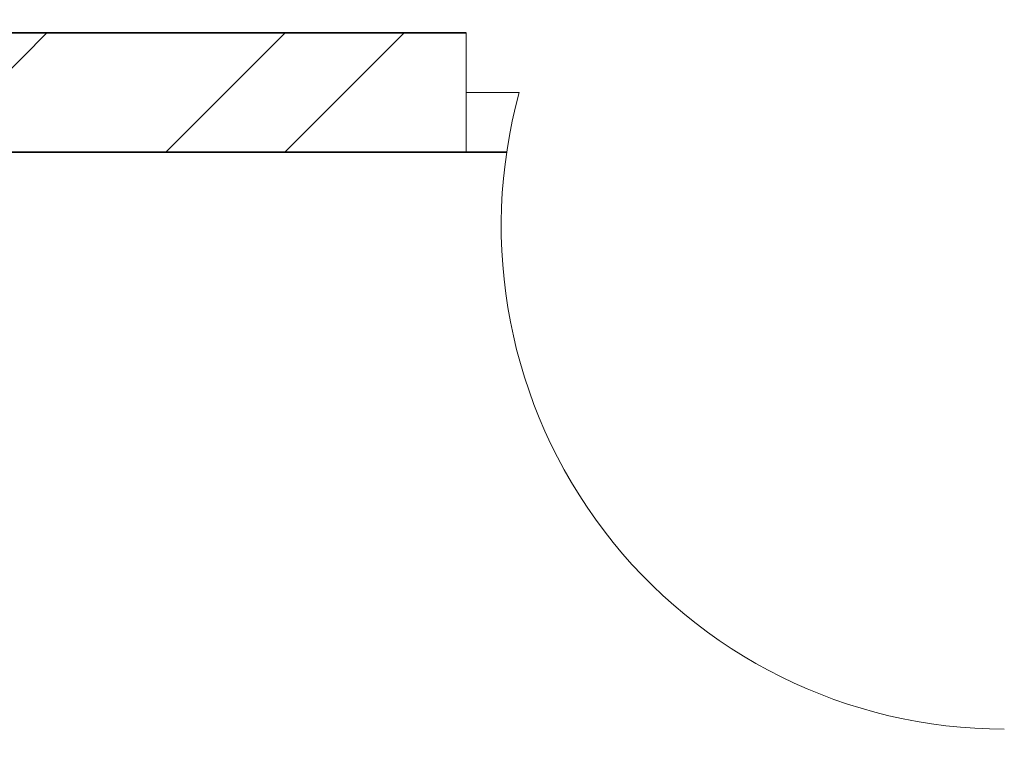
# Model space of a CAD drawing. Units: inches. Extents: x 1885 to 2748, y 783 to 2421.
# Tile 14 of 117: x 2065 to 2102, y 1065 to 1093. Entities that reach past the tile are written whole.
import ezdxf

# ---------------------------------------------------------------- set-up
doc = ezdxf.new("R2010")
doc.units = ezdxf.units.IN
doc.layers.add('A-DOOR', color=31, linetype='Continuous', lineweight=18)
doc.layers.add('A-WALL', color=7, linetype='Continuous', lineweight=35)
doc.layers.add('A-WALL-PATT', color=85, linetype='Continuous', lineweight=13, true_color=0x58ba48)

msp = doc.modelspace()

# ---------------------------------------------------------------- hatches: boundary and pattern name
at = {"layer": 'A-WALL-PATT'}
h = msp.add_hatch(dxfattribs=at)
h.set_pattern_fill('ANSI32', color=256)
h.paths.add_polyline_path([(2007.772, 2318.006), (1980.774, 2318.006), (1980.774, 2281.215), (1985.274, 2281.215), (1985.274, 2313.506), (2007.772, 2313.506), (2007.772, 2315.756)])
h.paths.add_polyline_path([(2094.324, 2318.006), (2067.772, 2318.006), (2067.772, 2313.506), (2094.324, 2313.506), (2094.324, 2315.756)])
h.paths.add_polyline_path([(2131.367, 2315.756), (2131.367, 2318.006), (2131.189, 2318.006), (2112.609, 2318.006), (2112.609, 2313.506), (2117.274, 2313.506), (2117.274, 2255.201), (2121.774, 2255.201), (2121.774, 2313.506), (2131.367, 2313.506)])
h.paths.add_polyline_path([(2190.512, 2318.006), (2155.367, 2318.006), (2155.367, 2313.506), (2169.774, 2313.506), (2169.774, 2229.506), (2121.774, 2229.506), (2121.774, 2233.451), (2119.524, 2233.451), (2117.274, 2233.451), (2117.274, 2201.101), (2121.774, 2201.101), (2121.774, 2225.006), (2169.774, 2225.006), (2169.774, 2165.006), (2306.274, 2165.006), (2306.274, 2066.006), (2310.774, 2066.006), (2344.274, 2066.006), (2486.274, 2066.006), (2486.274, 1886.006), (2483.02, 1886.006), (2483.02, 1881.506), (2486.274, 1881.506), (2486.274, 1880.678), (2490.774, 1880.678), (2490.774, 2070.506), (2344.274, 2070.506), (2310.774, 2070.506), (2310.774, 2165.006), (2310.774, 2173.636), (2308.524, 2173.636), (2306.274, 2173.636), (2306.274, 2169.506), (2174.274, 2169.506), (2174.274, 2313.506), (2190.512, 2313.506), (2190.512, 2315.756)])
h.paths.add_polyline_path([(1985.274, 2221.215), (1980.774, 2221.215), (1980.774, 2165.006), (1992.774, 2165.006), (1992.774, 2141.927), (1997.274, 2141.927), (1997.274, 2165.006), (2117.274, 2165.006), (2117.274, 2163.126), (2121.774, 2163.126), (2121.774, 2172.734), (2119.524, 2172.734), (2117.274, 2172.734), (2117.274, 2169.506), (1985.274, 2169.506)])
h.paths.add_polyline_path([(1997.274, 2105.927), (1992.774, 2105.927), (1992.774, 2070.506), (2016.774, 2070.506), (2016.774, 2059.123), (2019.024, 2059.123), (2021.274, 2059.123), (2021.274, 2070.506), (2117.274, 2070.506), (2117.274, 2022.506), (2114.423, 2022.506), (2114.423, 2018.006), (2123.627, 2018.006), (2123.627, 2020.256), (2123.627, 2022.506), (2121.774, 2022.506), (2121.774, 2142.587), (2119.524, 2142.587), (2117.274, 2142.587), (2117.274, 2075.006), (1997.274, 2075.006)])
h.paths.add_polyline_path([(2092.029, 2020.256), (2092.029, 2022.506), (2021.274, 2022.506), (2021.274, 2035.123), (2016.774, 2035.123), (2016.774, 2018.006), (2016.774, 1978.784), (2021.274, 1978.784), (2021.274, 2018.006), (2092.029, 2018.006)])
h.paths.add_polyline_path([(2260.938, 2022.506), (2153.105, 2022.506), (2153.105, 2020.256), (2153.105, 2018.006), (2155.274, 2018.006), (2155.274, 1886.006), (2107.629, 1886.006), (2107.629, 1881.506), (2182.911, 1881.506), (2182.911, 1883.756), (2182.911, 1886.006), (2159.774, 1886.006), (2159.774, 2018.006), (2260.938, 2018.006), (2260.938, 2020.256)])
h.paths.add_polyline_path([(2047.629, 1883.756), (2047.629, 1886.006), (2021.274, 1886.006), (2021.274, 1918.784), (2019.024, 1918.784), (2016.774, 1918.784), (2016.774, 1881.506), (2047.629, 1881.506)])
h.paths.add_polyline_path([(2306.361, 1883.756), (2306.361, 1886.006), (2296.274, 1886.006), (2296.274, 1982.006), (2316.535, 1982.006), (2316.535, 1984.256), (2316.535, 1986.506), (2296.274, 1986.506), (2296.274, 2022.506), (2289.276, 2022.506), (2289.276, 2018.006), (2291.774, 2018.006), (2291.774, 1886.006), (2242.911, 1886.006), (2242.911, 1881.506), (2306.361, 1881.506)], flags=17)
h.paths.add_polyline_path([(1985.274, 1843.006), (2021.6, 1843.006), (2021.534, 1845.441), (2021.477, 1847.506), (1980.774, 1847.506), (1980.774, 1809.446), (1985.274, 1809.446)])
h.paths.add_polyline_path([(2131.482, 1845.256), (2131.482, 1847.506), (2081.534, 1847.506), (2081.534, 1843.006), (2117.274, 1843.006), (2117.274, 1784.147), (2119.524, 1784.147), (2121.774, 1784.147), (2121.774, 1843.006), (2131.482, 1843.006)])
h.paths.add_polyline_path([(2203.886, 1847.506), (2155.482, 1847.506), (2155.482, 1843.006), (2169.774, 1843.006), (2169.774, 1759.006), (2121.774, 1759.006), (2121.774, 1761.457), (2117.274, 1761.457), (2117.274, 1730.429), (2121.774, 1730.429), (2121.774, 1754.506), (2177.421, 1754.506), (2177.421, 1756.756), (2177.421, 1759.006), (2174.274, 1759.006), (2174.274, 1843.006), (2203.886, 1843.006)])
h.paths.add_polyline_path([(2335.554, 1845.256), (2335.554, 1847.506), (2239.886, 1847.506), (2239.886, 1843.006), (2306.274, 1843.006), (2306.274, 1759.006), (2199.486, 1759.006), (2199.486, 1754.506), (2310.774, 1754.506), (2310.774, 1843.006), (2335.554, 1843.006)])
h.paths.add_polyline_path([(2348.774, 2022.506), (2344.274, 2022.506), (2344.274, 1986.506), (2341.681, 1986.506), (2341.681, 1982.006), (2344.274, 1982.006), (2344.274, 1886.006), (2330.361, 1886.006), (2330.361, 1881.506), (2361.627, 1881.506), (2361.627, 1883.756), (2361.627, 1886.006), (2348.774, 1886.006)], flags=17)
h.paths.add_polyline_path([(2283.251, 2315.756), (2283.251, 2318.006), (2238.512, 2318.006), (2238.512, 2313.506), (2283.251, 2313.506)], flags=17)
h.paths.add_polyline_path([(2363.274, 2348.006), (2388.677, 2348.006), (2388.677, 2350.256), (2388.677, 2352.506), (2358.774, 2352.506), (2358.774, 2348.006), (2358.774, 2318.006), (2344.481, 2318.006), (2344.481, 2313.506), (2358.774, 2313.506), (2358.774, 2229.506), (2310.774, 2229.506), (2310.774, 2231.952), (2306.274, 2231.952), (2306.274, 2205.611), (2310.774, 2205.611), (2310.774, 2225.006), (2358.774, 2225.006), (2358.774, 2211.506), (2452.329, 2211.506), (2452.329, 2213.756), (2452.329, 2216.006), (2363.274, 2216.006), (2363.274, 2318.006)])
h.paths.add_polyline_path([(2310.774, 2313.506), (2320.481, 2313.506), (2320.481, 2315.756), (2320.481, 2318.006), (2302.728, 2318.006), (2302.728, 2313.506), (2306.274, 2313.506), (2306.274, 2251.076), (2310.774, 2251.076)], flags=17)
h.paths.add_polyline_path([(2490.774, 2352.506), (2486.274, 2352.506), (2448.677, 2352.506), (2448.677, 2348.006), (2486.274, 2348.006), (2486.274, 2318.006), (2486.274, 2216.006), (2481.78, 2216.006), (2481.78, 2211.506), (2486.274, 2211.506), (2486.274, 2165.006), (2493.289, 2165.006), (2493.289, 2167.256), (2493.289, 2169.506), (2490.774, 2169.506), (2490.774, 2313.506), (2494.429, 2313.506), (2494.429, 2318.006), (2490.774, 2318.006)])
h.paths.add_polyline_path([(2534.653, 2318.006), (2515.691, 2318.006), (2515.691, 2313.506), (2534.653, 2313.506), (2534.653, 2315.756)])
h.paths.add_polyline_path([(2618.274, 2318.006), (2594.653, 2318.006), (2594.653, 2313.506), (2613.774, 2313.506), (2613.774, 2281.706), (2618.274, 2281.706)])
h.paths.add_polyline_path([(2618.274, 2221.706), (2613.774, 2221.706), (2613.774, 2169.506), (2554.019, 2169.506), (2554.019, 2165.006), (2613.774, 2165.006), (2613.774, 2152.878), (2618.274, 2152.878)])
h.paths.add_polyline_path([(2618.274, 2128.878), (2616.024, 2128.878), (2613.774, 2128.878), (2613.774, 2117.006), (2529.774, 2117.006), (2529.774, 2165.006), (2532.848, 2165.006), (2532.848, 2169.506), (2522.867, 2169.506), (2522.867, 2165.006), (2525.274, 2165.006), (2525.274, 2117.006), (2525.274, 2112.506), (2525.274, 2108.576), (2529.774, 2108.576), (2529.774, 2112.506), (2613.774, 2112.506), (2613.774, 2080.19), (2618.274, 2080.19)])
h.paths.add_polyline_path([(2618.274, 2044.19), (2616.024, 2044.19), (2613.774, 2044.19), (2613.774, 2015.506), (2529.774, 2015.506), (2529.774, 2088.582), (2527.524, 2088.582), (2525.274, 2088.582), (2525.274, 2011.006), (2613.774, 2011.006), (2613.774, 1956.755), (2618.274, 1956.755)])
h.paths.add_polyline_path([(2618.274, 1881.506), (2618.274, 1896.755), (2613.774, 1896.755), (2613.774, 1881.506), (2613.774, 1847.506), (2592.715, 1847.506), (2592.715, 1843.006), (2613.774, 1843.006), (2613.774, 1765.006), (2613.774, 1760.506), (2609.621, 1760.506), (2609.621, 1756.006), (2613.774, 1756.006), (2613.774, 1660.006), (2608.544, 1660.006), (2608.544, 1655.506), (2613.774, 1655.506), (2613.774, 1508.158), (2618.274, 1508.158)])
h.paths.add_polyline_path([(2565.774, 1843.006), (2568.997, 1843.006), (2568.997, 1847.506), (2490.774, 1847.506), (2490.774, 1849.7), (2488.524, 1849.7), (2486.274, 1849.7), (2486.274, 1847.506), (2477.274, 1847.506), (2477.274, 1838.506), (2477.274, 1821.493), (2486.274, 1821.493), (2486.274, 1838.506), (2561.274, 1838.506), (2561.274, 1765.006), (2486.274, 1765.006), (2486.274, 1786.157), (2477.274, 1786.157), (2477.274, 1765.006), (2477.274, 1756.006), (2486.274, 1756.006), (2565.774, 1756.006), (2585.621, 1756.006), (2585.621, 1758.256), (2585.621, 1760.506), (2565.774, 1760.506), (2565.774, 1765.006)])
h.paths.add_polyline_path([(2486.274, 1651.006), (2561.274, 1651.006), (2561.274, 1567.006), (2486.274, 1567.006), (2486.274, 1591.321), (2477.274, 1591.321), (2477.274, 1567.006), (2477.274, 1558.006), (2477.274, 1555.439), (2481.774, 1555.439), (2481.774, 1558.006), (2568.653, 1558.006), (2568.653, 1560.256), (2568.653, 1562.506), (2565.774, 1562.506), (2565.774, 1655.506), (2584.544, 1655.506), (2584.544, 1657.756), (2584.544, 1660.006), (2565.774, 1660.006), (2486.274, 1660.006), (2477.274, 1660.006), (2477.274, 1651.006), (2477.274, 1632.989), (2486.274, 1632.989)])
h.paths.add_polyline_path([(2449.967, 1883.756), (2449.967, 1886.006), (2421.627, 1886.006), (2421.627, 1881.506), (2449.967, 1881.506)], flags=17)
h.paths.add_polyline_path([(2447.274, 1847.506), (2395.554, 1847.506), (2395.554, 1843.006), (2442.774, 1843.006), (2442.774, 1809.27), (2447.274, 1809.27)])
h.paths.add_polyline_path([(1985.274, 1749.446), (1980.774, 1749.446), (1980.774, 1694.504), (1985.274, 1694.504), (1985.274, 1694.506), (1986.897, 1694.506), (1986.897, 1697.78), (1986.897, 1699.006), (1985.274, 1699.006)])
h.paths.add_polyline_path([(2152.774, 1699.006), (2121.774, 1699.006), (2121.774, 1703.668), (2119.524, 1703.668), (2117.274, 1703.668), (2117.274, 1699.006), (2009.219, 1699.006), (2009.219, 1694.506), (2148.274, 1694.506), (2148.274, 1692.631), (2152.774, 1692.631)])
h.paths.add_polyline_path([(2016.274, 1694.506), (2011.774, 1694.506), (2011.774, 1558.006), (2040.806, 1558.006), (2040.806, 1560.256), (2040.806, 1562.506), (2016.274, 1562.506)])
h.paths.add_polyline_path([(2152.774, 1663.017), (2150.524, 1663.017), (2148.274, 1663.017), (2148.274, 1562.506), (2100.806, 1562.506), (2100.806, 1558.006), (2165.119, 1558.006), (2165.119, 1560.256), (2165.119, 1562.506), (2152.774, 1562.506), (2152.774, 1610.506), (2224.774, 1610.506), (2224.774, 1607.99), (2229.274, 1607.99), (2229.274, 1615.006), (2152.774, 1615.006)])
h.paths.add_polyline_path([(2238.613, 1560.256), (2238.613, 1562.506), (2229.274, 1562.506), (2229.274, 1588.756), (2227.024, 1588.763), (2224.774, 1588.771), (2224.774, 1562.506), (2189.119, 1562.506), (2189.119, 1558.006), (2238.613, 1558.006)])
h.paths.add_polyline_path([(2336.024, 1560.256), (2336.024, 1562.506), (2310.774, 1562.506), (2310.774, 1656.347), (2308.524, 1656.347), (2306.274, 1656.347), (2306.274, 1562.506), (2286.613, 1562.506), (2286.613, 1558.006), (2336.024, 1558.006)])
h.paths.add_polyline_path([(2447.274, 1690.968), (2445.024, 1690.968), (2442.774, 1690.968), (2442.774, 1687.006), (2306.274, 1687.006), (2306.274, 1680.75), (2310.774, 1680.75), (2310.774, 1682.506), (2442.774, 1682.506), (2442.774, 1562.506), (2396.024, 1562.506), (2396.024, 1558.006), (2447.274, 1558.006)])
h.paths.add_polyline_path([(2447.274, 1749.27), (2445.024, 1749.27), (2442.774, 1749.27), (2442.774, 1717.232), (2447.274, 1717.232)])
h.paths.add_polyline_path([(2044.674, 1521.756), (2044.674, 1524.006), (2007.274, 1524.006), (2007.274, 1503.49), (2009.524, 1503.49), (2011.774, 1503.49), (2011.774, 1519.506), (2044.674, 1519.506)])
h.paths.add_polyline_path([(2177.969, 1521.756), (2177.969, 1524.006), (2104.674, 1524.006), (2104.674, 1519.506), (2145.774, 1519.506), (2145.774, 1387.506), (2143.37, 1387.506), (2143.37, 1383.006), (2251.585, 1383.006), (2251.585, 1385.256), (2251.585, 1387.506), (2150.274, 1387.506), (2150.274, 1519.506), (2177.969, 1519.506)])
h.paths.add_polyline_path([(2298.704, 1524.006), (2237.969, 1524.006), (2237.969, 1519.506), (2282.274, 1519.506), (2282.274, 1387.506), (2279.683, 1387.506), (2279.683, 1383.006), (2286.774, 1383.006), (2286.774, 1419.006), (2312.451, 1419.006), (2312.451, 1421.256), (2312.451, 1423.506), (2286.774, 1423.506), (2286.774, 1519.506), (2298.704, 1519.506), (2298.704, 1521.722)], flags=17)
h.paths.add_polyline_path([(2361.897, 1521.756), (2361.897, 1524.006), (2322.704, 1524.006), (2322.704, 1519.506), (2334.774, 1519.506), (2334.774, 1423.506), (2331.93, 1423.506), (2331.93, 1419.006), (2334.774, 1419.006), (2334.774, 1387.506), (2334.774, 1383.228), (2339.274, 1383.228), (2339.274, 1387.506), (2339.274, 1519.506), (2361.897, 1519.506)], flags=17)
h.paths.add_polyline_path([(2447.274, 1521.756), (2447.274, 1524.006), (2421.897, 1524.006), (2421.897, 1519.506), (2447.274, 1519.506)], flags=17)
h.paths.add_polyline_path([(2481.774, 1529.6), (2479.524, 1529.6), (2477.274, 1529.6), (2477.274, 1524.006), (2474.489, 1524.006), (2474.489, 1519.506), (2477.274, 1519.506), (2477.274, 1334.506), (2296.774, 1334.506), (2296.774, 1240.506), (2160.274, 1240.506), (2160.274, 1180.506), (2112.274, 1180.506), (2112.274, 1207.692), (2110.024, 1207.692), (2107.774, 1207.692), (2107.774, 1171.609), (2112.274, 1171.609), (2112.274, 1176.006), (2160.274, 1176.006), (2160.274, 1092.006), (2144.221, 1092.006), (2144.221, 1087.506), (2189.497, 1087.506), (2189.497, 1089.756), (2189.497, 1092.006), (2164.774, 1092.006), (2164.774, 1236.006), (2296.774, 1236.006), (2296.774, 1231.912), (2301.274, 1231.912), (2301.274, 1330.006), (2481.774, 1330.006), (2481.774, 1387.506)])
h.paths.add_polyline_path([(2618.274, 1448.158), (2613.774, 1448.158), (2613.774, 1382.506), (2529.774, 1382.506), (2525.274, 1382.506), (2525.274, 1307.062), (2529.774, 1307.062), (2529.774, 1378.006), (2613.774, 1378.006), (2613.774, 1354.988), (2618.274, 1354.988)])
h.paths.add_polyline_path([(2618.274, 1318.988), (2613.774, 1318.988), (2613.774, 1281.006), (2529.774, 1281.006), (2529.774, 1283.786), (2527.524, 1283.786), (2525.274, 1283.786), (2525.274, 1228.506), (2516.794, 1228.506), (2516.794, 1224.006), (2533.484, 1224.006), (2533.484, 1226.256), (2533.484, 1228.506), (2529.774, 1228.506), (2529.774, 1276.506), (2613.774, 1276.506), (2613.774, 1266.02), (2618.274, 1266.02)])
h.paths.add_polyline_path([(2618.274, 1134.964), (2613.774, 1134.964), (2613.774, 1092.006), (2594.545, 1092.006), (2594.545, 1087.506), (2618.274, 1087.506)])
h.paths.add_polyline_path([(2534.545, 1092.006), (2509.765, 1092.006), (2509.765, 1087.506), (2534.545, 1087.506), (2534.545, 1089.756)])
h.paths.add_polyline_path([(2481.274, 1224.006), (2484.117, 1224.006), (2484.117, 1226.256), (2484.117, 1228.506), (2476.774, 1228.506), (2476.774, 1198.506), (2471.61, 1198.506), (2471.61, 1194.006), (2476.774, 1194.006), (2476.774, 1062.006), (2436.894, 1062.006), (2436.894, 1057.506), (2476.774, 1057.506), (2481.274, 1057.506), (2481.274, 1062.006), (2481.274, 1087.506), (2485.354, 1087.506), (2485.354, 1089.756), (2485.354, 1092.006), (2481.274, 1092.006), (2481.274, 1117.506)])
h.paths.add_polyline_path([(2439.898, 1198.506), (2349.274, 1198.506), (2349.274, 1194.006), (2349.274, 1180.506), (2301.274, 1180.506), (2301.274, 1201.896), (2299.024, 1201.896), (2296.774, 1201.896), (2296.774, 1172.335), (2299.024, 1172.335), (2301.274, 1172.335), (2301.274, 1176.006), (2349.274, 1176.006), (2349.274, 1092.006), (2334.452, 1092.006), (2334.452, 1087.506), (2349.274, 1087.506), (2349.274, 1057.506), (2353.774, 1057.506), (2376.894, 1057.506), (2376.894, 1059.756), (2376.894, 1062.006), (2353.774, 1062.006), (2353.774, 1087.506), (2353.774, 1180.506), (2353.774, 1194.006), (2439.898, 1194.006), (2439.898, 1196.256)])
h.paths.add_polyline_path([(2270.596, 1089.756), (2270.596, 1092.006), (2249.497, 1092.006), (2249.497, 1087.506), (2270.596, 1087.506)], flags=17)
h.paths.add_polyline_path([(2310.452, 1092.006), (2301.274, 1092.006), (2301.274, 1153.292), (2296.774, 1153.292), (2296.774, 1092.006), (2293.786, 1092.006), (2293.786, 1087.506), (2310.452, 1087.506), (2310.452, 1089.756)], flags=17)
h.paths.add_polyline_path([(2112.274, 1150.328), (2110.024, 1150.328), (2107.774, 1150.328), (2107.774, 1092.006), (2104.465, 1092.006), (2104.465, 1087.506), (2120.221, 1087.506), (2120.221, 1089.756), (2120.221, 1092.006), (2112.274, 1092.006)])
h.paths.add_polyline_path([(2082.172, 1092.006), (2058.144, 1092.006), (2058.144, 1087.506), (2082.172, 1087.506), (2082.172, 1089.756)])
h.paths.add_polyline_path([(1975.774, 1145.638), (1971.274, 1145.638), (1971.274, 1087.506), (1980.774, 1087.506), (1998.144, 1087.506), (1998.144, 1089.756), (1998.144, 1092.006), (1985.274, 1092.006), (1975.774, 1092.006)])
h.paths.add_polyline_path([(2112.274, 1244.385), (2110.024, 1244.385), (2107.774, 1244.385), (2107.774, 1240.506), (1992.274, 1240.506), (1992.274, 1271.008), (1987.774, 1271.008), (1987.774, 1240.506), (1980.774, 1240.506), (1975.774, 1240.506), (1971.274, 1240.506), (1971.274, 1205.638), (1975.774, 1205.638), (1975.774, 1236.006), (2107.774, 1236.006), (2107.774, 1233.444), (2112.274, 1233.444), (2112.274, 1236.006)])
h.paths.add_polyline_path([(2112.274, 1383.006), (2114.783, 1383.006), (2114.783, 1385.256), (2114.783, 1387.506), (2102.476, 1387.506), (2102.476, 1383.006), (2107.774, 1383.006), (2107.774, 1335.006), (2011.774, 1335.006), (2011.774, 1349.939), (2007.274, 1349.939), (2007.274, 1335.006), (1987.774, 1335.006), (1987.774, 1330.506), (1987.774, 1307.008), (1992.274, 1307.008), (1992.274, 1330.506), (2007.274, 1330.506), (2107.774, 1330.506), (2107.774, 1264.711), (2112.274, 1264.711)])
h.paths.add_polyline_path([(2077.857, 1387.506), (2011.774, 1387.506), (2011.774, 1390.036), (2009.524, 1390.036), (2007.274, 1390.036), (2007.274, 1373.939), (2011.774, 1373.939), (2011.774, 1383.006), (2077.857, 1383.006)])
h.paths.add_polyline_path([(2011.774, 1443.49), (2007.274, 1443.49), (2007.274, 1410.248), (2011.774, 1410.248)])

# ---------------------------------------------------------------- linework, layer by layer
at = {"layer": 'A-DOOR'}
for p, q in [((2082.172, 1092.006), (2082.172, 1087.506)), ((2082.172, 1087.506), (2082.172, 1089.756)), ((2082.172, 1089.756), (2084.172, 1089.756))]:
    msp.add_line(p, q, dxfattribs=at)
msp.add_arc((2102.465, 1084.728), 18.972, 164.6316, 270, dxfattribs=at)
at = {"layer": 'A-WALL'}
for p, q in [((2082.172, 1092.006), (2058.144, 1092.006)), ((2083.698, 1087.506), (2058.144, 1087.506))]:
    msp.add_line(p, q, dxfattribs=at)

doc.saveas('drawing.dxf')
